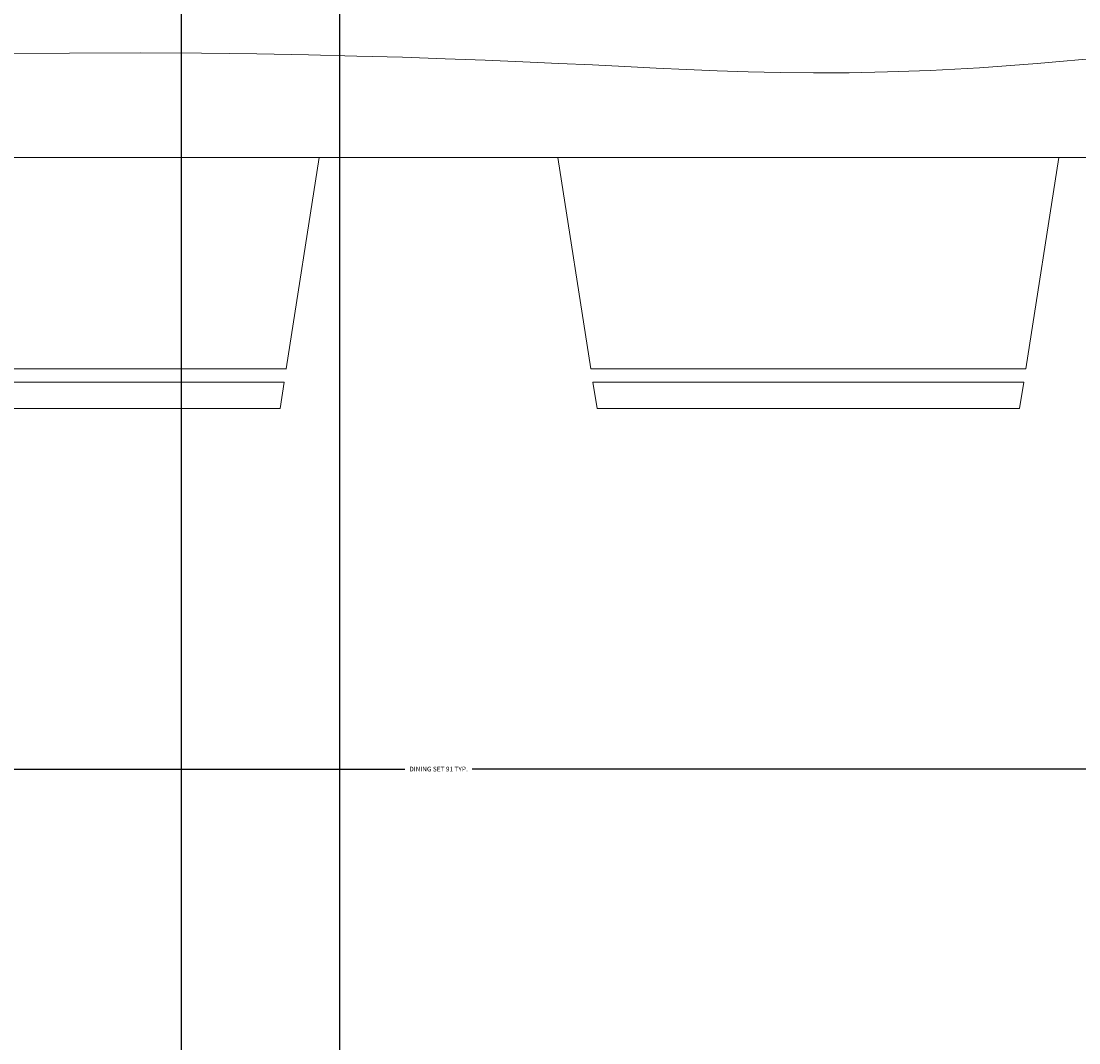
# Model space of a CAD drawing. Units: inches. Extents: x 7359 to 7979, y 33027 to 34263.
# Tile 7 of 32: x 7688 to 7728, y 33347 to 33386. Entities that reach past the tile are written whole.
import ezdxf

# ---------------------------------------------------------------- set-up
doc = ezdxf.new("R2010")
doc.units = ezdxf.units.IN
doc.layers.add('A-ANNO-DIMS', color=2, linetype='Continuous', lineweight=18)
doc.layers.add('A-FURN', color=8, linetype='Continuous', lineweight=18)
doc.styles.get("Standard").update_dxf_attribs({"font": 'arial.ttf'})
doc.dimstyles.get("Standard").update_dxf_attribs({"dimtxt": 0.18, "dimasz": 0.18, "dimexe": 0.18, "dimexo": 0.0625, "dimgap": 0.09, "dimtad": 0, "dimtih": 1, "dimtoh": 1, "dimdec": 4, "dimzin": 0, "dimdsep": 46, "dimtxsty": 'Standard', "dimcen": 0.09, "dimadec": 0, "dimazin": 0, "dimtfac": 1, "dimtdec": 4, "dimtofl": 0, "dimtmove": 0, "dimatfit": 3, "dimfxl": 1, "dimtolj": 1, "dimtzin": 0, "dimarcsym": 0})

# ---------------------------------------------------------------- blocks, each defined once
blk = doc.blocks.new('Dining Set - 36 x 72 in.')
for p, q in [((-36, -18), (36, -18)), ((-4.5152, -17.99762), (-5.7655, -25.99928)), ((5.7657, -26.0006), (4.5153, -17.99762)), ((23.4848, -17.99762), (22.2345, -25.99928)), ((-22.2304, -26), (-5.7608, -26)), ((5.7696, -26), (22.2392, -26)), ((-5.8416, -26.5), (-22.1534, -26.5)), ((-5.8437, -26.49967), (-6, -27.5)), ((6, -27.5), (5.8438, -26.50044)), ((22.1584, -26.5), (5.8466, -26.5)), ((22.1563, -26.49967), (22, -27.5)), ((-22, -27.5), (-6, -27.5)), ((6, -27.5), (22, -27.5))]:
    blk.add_line(p, q)
blk.add_lwpolyline([(-17.0781, -14.07292), (-13.97, -14.04671), (-11.3027, -14.04297), (-8.9724, -14.05681), (-6.875, -14.08334), (-4.9224, -14.11833), (-3.0905, -14.16016), (-1.3709, -14.20785), (0.2448, -14.26042), (1.7647, -14.3169), (3.1973, -14.3763), (4.5507, -14.43767), (5.8333, -14.5), (7.0554, -14.5621), (8.235, -14.62175), (9.3922, -14.67652), (10.5469, -14.72396), (11.7192, -14.76164), (12.929, -14.78711), (14.1965, -14.79794), (15.5417, -14.79167), (16.9933, -14.76424), (18.6152, -14.70508), (20.4804, -14.60197), (22.6615, -14.44271), (25.2312, -14.21509)])
blk = doc.blocks.new('*D36')
at = {"layer": 'A-ANNO-DIMS', "color": 0, "lineweight": -2, "transparency": 16777216}
for p, q in [((7657.863, 33371.281), (7657.863, 33357.514)), ((7748.863, 33371.281), (7748.863, 33357.514)), ((7658.043, 33357.694), (7702.085, 33357.694)), ((7748.683, 33357.694), (7704.641, 33357.694))]:
    blk.add_line(p, q, dxfattribs=at)
at = {"layer": 'A-ANNO-DIMS', "color": 0, "transparency": 16777216}
for points in [[(7658.043, 33357.724), (7658.043, 33357.664), (7657.863, 33357.694)], [(7748.683, 33357.724), (7748.683, 33357.664), (7748.863, 33357.694)]]:
    blk.add_solid(points, dxfattribs=at)
at = {"layer": 'Defpoints', "color": 0, "transparency": 16777216}
for p in [(7657.863, 33371.344), (7748.863, 33371.344), (7748.863, 33357.694)]:
    blk.add_point(p, dxfattribs=at)
at = {"layer": 'A-ANNO-DIMS', "color": 0, "transparency": 16777216, "insert": (7703.363, 33357.694), "char_height": 0.18, "attachment_point": 5}
blk.add_mtext('\\A1;DINING SET 91 TYP.', dxfattribs=at)
blk = doc.blocks.new('*D89')
at = {"layer": 'A-ANNO-DIMS', "color": 0, "lineweight": -2, "transparency": 16777216}
for p, q in [((7693.626578, 33301.124789), (7693.626578, 33657.242289)), ((7699.626578, 33301.124789), (7699.626578, 33657.242289)), ((7693.806578, 33657.062289), (7696.477151, 33657.062289)), ((7699.446578, 33657.062289), (7696.776005, 33657.062289))]:
    blk.add_line(p, q, dxfattribs=at)
at = {"layer": 'A-ANNO-DIMS', "color": 0, "transparency": 16777216}
for points in [[(7693.806578, 33657.092289), (7693.806578, 33657.032289), (7693.626578, 33657.062289)], [(7699.446578, 33657.092289), (7699.446578, 33657.032289), (7699.626578, 33657.062289)]]:
    blk.add_solid(points, dxfattribs=at)
at = {"layer": 'Defpoints', "color": 0, "transparency": 16777216}
for p in [(7699.626578, 33657.062289), (7693.626578, 33301.062289), (7699.626578, 33301.062289)]:
    blk.add_point(p, dxfattribs=at)
at = {"layer": 'A-ANNO-DIMS', "color": 0, "transparency": 16777216, "insert": (7696.626578, 33657.062289), "char_height": 0.18, "attachment_point": 5}
blk.add_mtext('\\A1;6', dxfattribs=at)

msp = doc.modelspace()

# ---------------------------------------------------------------- block references
at = {"layer": 'A-FURN'}
msp.add_blockref('Dining Set - 36 x 72 in.', (7703.363, 33398.8436), dxfattribs=at)

# ---------------------------------------------------------------- dimensions: what is measured, and where the dimension line sits
at = {"layer": 'A-ANNO-DIMS'}
dim = msp.add_linear_dim(base=(7699.6266, 33657.0623), p1=(7693.6266, 33301.0623), p2=(7699.6266, 33301.0623), dimstyle='Standard', override={"dimdec": 0, "dimlfac": 1, "dimrnd": 0, "dimzin": 0, "dimdsep": 46, "dimlunit": 2}, dxfattribs=at)
dim.commit()
dim.dimension.update_dxf_attribs({"geometry": '*D89', "text_midpoint": (7696.6266, 33657.0623)})
dim = msp.add_linear_dim(base=(7748.863, 33357.6936), p1=(7657.863, 33371.3436), p2=(7748.863, 33371.3436), text='DINING SET <> TYP.', dimstyle='Standard', override={"dimdec": 0, "dimlfac": 1, "dimrnd": 0, "dimzin": 0, "dimdsep": 46, "dimlunit": 2}, dxfattribs=at)
dim.commit()
dim.dimension.update_dxf_attribs({"geometry": '*D36', "text_midpoint": (7703.363, 33357.6936)})

doc.saveas('drawing.dxf')
